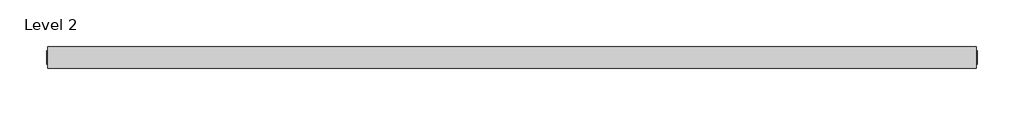
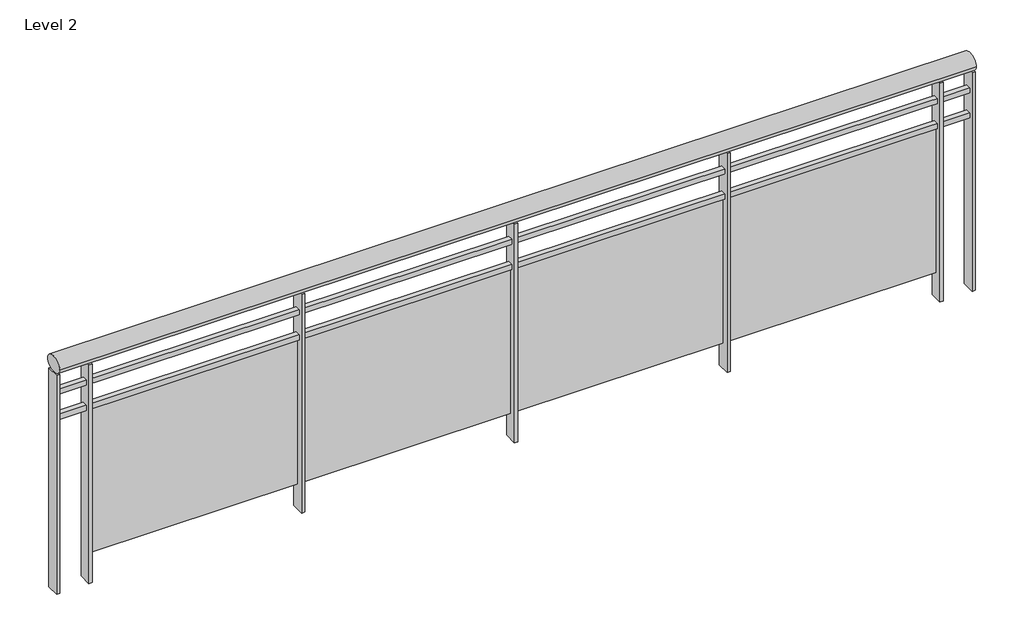
# One storey: 1 railing.
"""IFC4 building model written with IfcOpenShell, lengths in millimetres."""

from ifc_helpers import new_model, si_unit, point, frame, origin, place, context, project, spatial, polyline, ellipse_curve, trimmed, outline, extrude, element, save
from ifc_brep_helpers import plane_surface, extruded_surface, advanced_brep

model = new_model("IFC4")

# Units and contexts
model_context = context("Model", 3, world=origin())
ifc_project = project(units=[si_unit("LENGTHUNIT", "METRE", prefix="MILLI")], contexts=[model_context])

# Site, building, storey
site = spatial("IfcSite", under=ifc_project)
building = spatial("IfcBuilding", under=site)
storey = spatial("IfcBuildingStorey", under=building, Name="Level 2", Elevation=6096.0)

# Railing
placement = place(None, origin())
element("IfcRailing", 1, ObjectType="Glass Panel - Bottom Fill", at=placement, inside=storey, context=model_context, shape_type="SolidModel", body=[
    advanced_brep(
    [(-3870.2434506, -20475.1117988, 4567.9552714), (-3870.2434506, -20395.1117988, 4567.9552714), (-7316.7383357, -20475.1117988, 4567.9552714), (-7316.7383357, -20395.1117988, 4567.9552714)],
    [
        (0, 1, ellipse_curve(frame((-3870.2434506, -20435.1117988, 4567.9552714), z_axis=(1.0, 0.0, 0.0), x_axis=(0.0, 1.0, 0.0)), 40.0, 30.0)),
        (1, 0, ellipse_curve(frame((-3870.2434506, -20435.1117988, 4567.9552714), z_axis=(1.0, 0.0, 0.0), x_axis=(0.0, 1.0, 0.0)), 40.0, 30.0)),
        (2, 3, ellipse_curve(frame((-7316.7383357, -20435.1117988, 4567.9552714), z_axis=(-1.0, 0.0, 0.0), x_axis=(0.0, 1.0, 0.0)), 40.0, 30.0)),
        (3, 2, ellipse_curve(frame((-7316.7383357, -20435.1117988, 4567.9552714), z_axis=(-1.0, 0.0, 0.0), x_axis=(0.0, 1.0, 0.0)), 40.0, 30.0)),
        (1, 3),
        (2, 0),
    ],
    [
        plane_surface(frame((-3870.2434506, -20435.1117988, 4567.9552714), z_axis=(1.0, 0.0, 0.0), x_axis=(0.0, -1.0, 0.0))),
        plane_surface(frame((-7316.7383357, -20435.1117988, 4567.9552714), z_axis=(-1.0, 0.0, 0.0), x_axis=(0.0, -1.0, 0.0))),
        extruded_surface(trimmed(ellipse_curve(frame((-7316.7383357, -20435.1117988, 4567.9552714), z_axis=(1.0, 0.0, 0.0), x_axis=(0.0, 1.0, 0.0)), 40.0, 30.0), [point((-7316.7383357, -20395.1117988, 4567.9552714))], [point((-7316.7383357, -20475.1117988, 4567.9552714))], True, "CARTESIAN"), (3446.4948851, 0.0, 0.0), 3446.4948851),
        extruded_surface(trimmed(ellipse_curve(frame((-7316.7383357, -20435.1117988, 4567.9552714), z_axis=(1.0, 0.0, 0.0), x_axis=(0.0, 1.0, 0.0)), 40.0, 30.0), [point((-7316.7383357, -20475.1117988, 4567.9552714))], [point((-7316.7383357, -20395.1117988, 4567.9552714))], True, "CARTESIAN"), (3446.4948851, 0.0, 0.0), 3446.4948851),
    ],
    [
        (0, [[1, 2]]),
        (1, [[3, 4]]),
        (2, [[-2, 5, -3, 6]]),
        (3, [[-1, -6, -4, -5]]),
    ],
),
    extrude(outline(polyline([(-3870.2434506, -20425.7210337), (-3870.2434506, -20445.7210337), (-7316.7383357, -20445.7210337), (-7316.7383357, -20425.7210337), (-3870.2434506, -20425.7210337)])), frame((0.0, 0.0, 4447.9552714), z_axis=(0.0, 0.0, 1.0), x_axis=(1.0, 0.0, 0.0)), (0.0, 0.0, 1.0), 20.0),
    extrude(outline(polyline([(-3870.2434506, -20425.7210337), (-3870.2434506, -20445.7210337), (-7316.7383357, -20445.7210337), (-7316.7383357, -20425.7210337), (-3870.2434506, -20425.7210337)])), frame((0.0, 0.0, 4347.9552714), z_axis=(0.0, 0.0, 1.0), x_axis=(1.0, 0.0, 0.0)), (0.0, 0.0, 1.0), 20.0),
    extrude(outline(polyline([(-7187.4908931, -20460.7210337), (-7199.4908931, -20460.7210337), (-7199.4908931, -20410.7210337), (-7187.4908931, -20410.7210337), (-7187.4908931, -20460.7210337)])), frame((0.0, 0.0, 3667.9552714), z_axis=(0.0, 0.0, 1.0), x_axis=(1.0, 0.0, 0.0)), (0.0, 0.0, 1.0), 869.8465326),
    extrude(outline(polyline([(-6393.4908931, -20433.9962236), (-7193.4908931, -20433.9962236), (-7193.4908931, -20428.9962236), (-6393.4908931, -20428.9962236), (-6393.4908931, -20433.9962236)])), frame((0.0, 0.0, 3767.9552714), z_axis=(0.0, 0.0, 1.0), x_axis=(1.0, 0.0, 0.0)), (0.0, 0.0, 1.0), 580.0),
    extrude(outline(polyline([(-6387.4908931, -20460.7210337), (-6399.4908931, -20460.7210337), (-6399.4908931, -20410.7210337), (-6387.4908931, -20410.7210337), (-6387.4908931, -20460.7210337)])), frame((0.0, 0.0, 3667.9552714), z_axis=(0.0, 0.0, 1.0), x_axis=(1.0, 0.0, 0.0)), (0.0, 0.0, 1.0), 869.8465326),
    extrude(outline(polyline([(-5593.4908931, -20433.9962236), (-6393.4908931, -20433.9962236), (-6393.4908931, -20428.9962236), (-5593.4908931, -20428.9962236), (-5593.4908931, -20433.9962236)])), frame((0.0, 0.0, 3767.9552714), z_axis=(0.0, 0.0, 1.0), x_axis=(1.0, 0.0, 0.0)), (0.0, 0.0, 1.0), 580.0),
    extrude(outline(polyline([(-5587.4908931, -20460.7210337), (-5599.4908931, -20460.7210337), (-5599.4908931, -20410.7210337), (-5587.4908931, -20410.7210337), (-5587.4908931, -20460.7210337)])), frame((0.0, 0.0, 3667.9552714), z_axis=(0.0, 0.0, 1.0), x_axis=(1.0, 0.0, 0.0)), (0.0, 0.0, 1.0), 869.8465326),
    extrude(outline(polyline([(-4793.4908931, -20433.9962236), (-5593.4908931, -20433.9962236), (-5593.4908931, -20428.9962236), (-4793.4908931, -20428.9962236), (-4793.4908931, -20433.9962236)])), frame((0.0, 0.0, 3767.9552714), z_axis=(0.0, 0.0, 1.0), x_axis=(1.0, 0.0, 0.0)), (0.0, 0.0, 1.0), 580.0),
    extrude(outline(polyline([(-4787.4908931, -20460.7210337), (-4799.4908931, -20460.7210337), (-4799.4908931, -20410.7210337), (-4787.4908931, -20410.7210337), (-4787.4908931, -20460.7210337)])), frame((0.0, 0.0, 3667.9552714), z_axis=(0.0, 0.0, 1.0), x_axis=(1.0, 0.0, 0.0)), (0.0, 0.0, 1.0), 869.8465326),
    extrude(outline(polyline([(-3993.4908931, -20433.9962236), (-4793.4908931, -20433.9962236), (-4793.4908931, -20428.9962236), (-3993.4908931, -20428.9962236), (-3993.4908931, -20433.9962236)])), frame((0.0, 0.0, 3767.9552714), z_axis=(0.0, 0.0, 1.0), x_axis=(1.0, 0.0, 0.0)), (0.0, 0.0, 1.0), 580.0),
    extrude(outline(polyline([(-3987.4908931, -20460.7210337), (-3999.4908931, -20460.7210337), (-3999.4908931, -20410.7210337), (-3987.4908931, -20410.7210337), (-3987.4908931, -20460.7210337)])), frame((0.0, 0.0, 3667.9552714), z_axis=(0.0, 0.0, 1.0), x_axis=(1.0, 0.0, 0.0)), (0.0, 0.0, 1.0), 869.8465326),
    extrude(outline(polyline([(-7308.7383357, -20460.7210337), (-7320.7383357, -20460.7210337), (-7320.7383357, -20410.7210337), (-7308.7383357, -20410.7210337), (-7308.7383357, -20460.7210337)])), frame((0.0, 0.0, 3667.9552714), z_axis=(0.0, 0.0, 1.0), x_axis=(1.0, 0.0, 0.0)), (0.0, 0.0, 1.0), 869.8465326),
    extrude(outline(polyline([(-3866.2434506, -20460.7210337), (-3878.2434506, -20460.7210337), (-3878.2434506, -20410.7210337), (-3866.2434506, -20410.7210337), (-3866.2434506, -20460.7210337)])), frame((0.0, 0.0, 3667.9552714), z_axis=(0.0, 0.0, 1.0), x_axis=(1.0, 0.0, 0.0)), (0.0, 0.0, 1.0), 869.8465326),
])

save(model, "model.ifc")

# Revit data of these elements
# Type "Glass Panel - Bottom Fill"
#   built-in parameter 1008612 = 0.019685 (stored number, unit not read)
#   built-in parameter 1008611 = 0.019685 (stored number, unit not read)
#   built-in parameter 1008609 = 0.902231 (stored number, unit not read)
#   built-in parameter 1008604 = 0.19685 (stored number, unit not read)
#   built-in parameter 1008603 = 0.164042 (stored number, unit not read)
#   Railing Height = 2' - 11.43307"
#   built-in parameter 1008630 = 2
#   built-in parameter 1008610 = 2
# Element 1 (IfcRailing, "Glass Panel - Bottom Fill")
#   built-in parameter 1008621 = -7.96603 (stored number, unit not read)
#   Phase Created = New Construction
#   Materials on its faces: "Metal - Stainless Steel,Polished", "Glass"
# Materials
#   "Metal - Stainless Steel,Polished": class "Metal", colour RGB 189 187 185, transparency 0, Cost = 0
#   "Glass": class "Glass", colour RGB 218 227 224, transparency 0.85, Description = "Soda Lime Glass", Cost = 0
